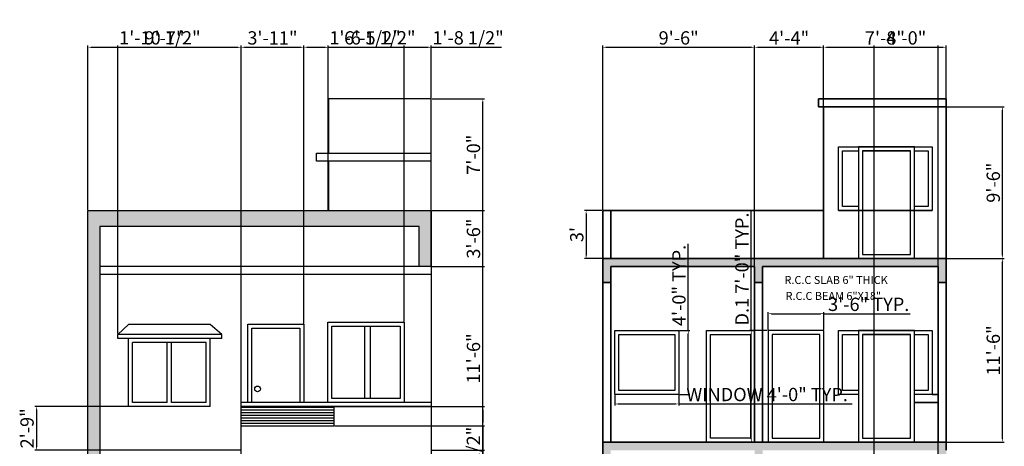
# Model space of a CAD drawing. Units: inches. Extents: x 2368 to 3882, y 1243 to 2139.
# Tile 6 of 6: x 3100 to 3840, y 1745 to 2065. Entities that reach past the tile are written whole.
import ezdxf

# ---------------------------------------------------------------- set-up
doc = ezdxf.new("R2010")
doc.units = ezdxf.units.IN
for name, color, linetype, lineweight in [('A-ANNO-DIMS', 2, 'Continuous', 18), ('A-ANNO-TEXT', 7, 'Continuous', 18), ('A-ELEV', 7, 'Continuous', 25), ('A-ELEV-PATT', 252, 'Continuous', 13), ('A-SECT', 7, 'Continuous', 35), ('A-SECT-PATT', 8, 'Continuous', 13)]:
    doc.layers.add(name, color=color, linetype=linetype, lineweight=lineweight)
doc.styles.get("Standard").update_dxf_attribs({"font": 'arial.ttf'})
doc.dimstyles.new('ISO-25', dxfattribs={"dimtxt": 10, "dimasz": 2.5, "dimexe": 1.25, "dimexo": 0.625, "dimtad": 1, "dimlunit": 3, "dimtxsty": 'Standard', "dimcen": 2.5, "dimadec": 0, "dimazin": 0, "dimtfac": 1, "dimtmove": 0, "dimatfit": 3, "dimfxl": 1, "dimarcsym": 0})

# ---------------------------------------------------------------- blocks, each defined once
blk = doc.blocks.new('*D13')
at = {"layer": 'A-ANNO-DIMS', "color": 0, "lineweight": -2, "transparency": 16777216}
for p, q in [((3537.71, 1921.84), (3524.56, 1921.84)), ((3525.81, 1919.34), (3525.81, 1888.34)), ((3537.71, 1885.84), (3524.56, 1885.84))]:
    blk.add_line(p, q, dxfattribs=at)
at = {"layer": 'A-ANNO-DIMS', "color": 0, "transparency": 16777216}
for points in [[(3525.39, 1919.34), (3526.22, 1919.34), (3525.81, 1921.84)], [(3525.39, 1888.34), (3526.22, 1888.34), (3525.81, 1885.84)]]:
    blk.add_solid(points, dxfattribs=at)
at = {"layer": 'Defpoints', "color": 0, "transparency": 16777216}
for p in [(3538.34, 1921.84), (3525.81, 1885.84), (3538.34, 1885.84)]:
    blk.add_point(p, dxfattribs=at)
at = {"layer": 'A-ANNO-DIMS', "color": 0, "transparency": 16777216, "insert": (3520.07, 1903.84), "char_height": 10, "attachment_point": 5, "rotation": 90}
blk.add_mtext("3'", dxfattribs=at)
blk = doc.blocks.new('WIN-ELEV-CHAJJA')
for p, q in [((3166.48, 1408.84), (3174.49, 1416.36)), ((3235.8, 1416.36), (3174.49, 1416.36)), ((3244.48, 1408.84), (3235.8, 1416.36)), ((3244.48, 1408.84), (3166.48, 1408.84)), ((3166.48, 1405.84), (3166.48, 1408.84)), ((3244.48, 1405.84), (3166.48, 1405.84)), ((3174.49, 1354.84), (3174.49, 1405.84)), ((3235.8, 1354.84), (3235.8, 1405.84)), ((3244.48, 1405.84), (3244.48, 1408.84)), ((3232.8, 1402.84), (3177.49, 1402.84)), ((3177.49, 1357.84), (3177.49, 1402.84)), ((3203.49, 1357.84), (3203.49, 1402.84)), ((3206.8, 1357.84), (3206.8, 1402.84)), ((3232.8, 1357.84), (3232.8, 1402.84)), ((3235.8, 1354.84), (3174.49, 1354.84)), ((3203.49, 1357.84), (3177.49, 1357.84)), ((3232.8, 1357.84), (3206.8, 1357.84))]:
    blk.add_line(p, q)
blk = doc.blocks.new('DOOR-ELEV')
for p, q in [((3271.73, 1507.84), (3271.73, 1566.55)), ((3271.73, 1566.55), (3313.73, 1566.55)), ((3274.73, 1507.84), (3274.73, 1563.55)), ((3274.73, 1563.55), (3310.73, 1563.55)), ((3310.73, 1563.55), (3310.73, 1507.84)), ((3313.73, 1566.55), (3313.73, 1507.84))]:
    blk.add_line(p, q)
blk.add_circle((3278.95, 1517.95), 2.15)
blk = doc.blocks.new('WIN-SECT-SQ')
for points in [[(3547.39, 1831.84), (3595.39, 1831.84), (3595.39, 1783.84), (3547.39, 1783.84)], [(3550.39, 1828.84), (3592.39, 1828.84), (3592.39, 1786.84), (3550.39, 1786.84)]]:
    blk.add_lwpolyline(points, close=True)
blk = doc.blocks.new('DOOR-SECT')
for points in [[(3662.52, 1747.84), (3704.52, 1747.84), (3704.52, 1831.84), (3662.52, 1831.84)], [(3665.52, 1750.84), (3701.52, 1750.84), (3701.52, 1828.84), (3665.52, 1828.84)]]:
    blk.add_lwpolyline(points, close=True)
blk = doc.blocks.new('DOOR-SECT-2')
for points in [[(3652.34, 1471.84), (3616.34, 1471.84), (3616.34, 1555.84), (3652.34, 1555.84)], [(3649.34, 1474.84), (3619.34, 1474.84), (3619.34, 1552.84), (3649.34, 1552.84)]]:
    blk.add_lwpolyline(points, close=True)
blk = doc.blocks.new('WIN-DOOR-SECT')
for points in [[(3730.54, 1783.84), (3715.45, 1783.84), (3715.45, 1831.84), (3785.77, 1831.84), (3785.77, 1783.84), (3772.54, 1783.84)], [(3730.54, 1786.84), (3718.45, 1786.84), (3718.45, 1828.84), (3730.54, 1828.84)], [(3733.54, 1828.84), (3769.54, 1828.84)], [(3772.54, 1828.84), (3782.77, 1828.84), (3782.77, 1786.84), (3772.54, 1786.84)]]:
    blk.add_lwpolyline(points)
for points in [[(3730.54, 1747.84), (3772.54, 1747.84), (3772.54, 1831.84), (3730.54, 1831.84)], [(3733.54, 1750.84), (3769.54, 1750.84), (3769.54, 1828.84), (3733.54, 1828.84)]]:
    blk.add_lwpolyline(points, close=True)
blk = doc.blocks.new('*D26')
at = {"layer": 'A-ANNO-DIMS', "color": 0, "lineweight": -2, "transparency": 16777216}
for p, q in [((3547.39, 1783.21), (3547.39, 1775.39)), ((3595.39, 1783.21), (3595.39, 1775.39)), ((3549.89, 1776.64), (3592.89, 1776.64)), ((3595.39, 1776.64), (3725.68, 1776.64))]:
    blk.add_line(p, q, dxfattribs=at)
at = {"layer": 'A-ANNO-DIMS', "color": 0, "transparency": 16777216}
for points in [[(3549.89, 1777.05), (3549.89, 1776.22), (3547.39, 1776.64)], [(3592.89, 1777.05), (3592.89, 1776.22), (3595.39, 1776.64)]]:
    blk.add_solid(points, dxfattribs=at)
at = {"layer": 'Defpoints', "color": 0, "transparency": 16777216}
for p in [(3547.39, 1783.84), (3595.39, 1783.84), (3595.39, 1776.64)]:
    blk.add_point(p, dxfattribs=at)
at = {"layer": 'A-ANNO-DIMS', "color": 0, "transparency": 16777216, "insert": (3661.79, 1782.44), "char_height": 10, "attachment_point": 5}
blk.add_mtext('WINDOW 4\'-0" TYP.', dxfattribs=at)
blk = doc.blocks.new('*D27')
at = {"layer": 'A-ANNO-DIMS', "color": 0, "lineweight": -2, "transparency": 16777216}
for p, q in [((3602.59, 1831.84), (3602.59, 1896.95)), ((3596.02, 1831.84), (3603.84, 1831.84)), ((3602.59, 1786.34), (3602.59, 1829.34)), ((3596.02, 1783.84), (3603.84, 1783.84))]:
    blk.add_line(p, q, dxfattribs=at)
at = {"layer": 'A-ANNO-DIMS', "color": 0, "transparency": 16777216}
for points in [[(3602.18, 1829.34), (3603.01, 1829.34), (3602.59, 1831.84)], [(3602.18, 1786.34), (3603.01, 1786.34), (3602.59, 1783.84)]]:
    blk.add_solid(points, dxfattribs=at)
at = {"layer": 'Defpoints', "color": 0, "transparency": 16777216}
for p in [(3595.39, 1831.84), (3602.59, 1831.84), (3595.39, 1783.84)]:
    blk.add_point(p, dxfattribs=at)
at = {"layer": 'A-ANNO-DIMS', "color": 0, "transparency": 16777216, "insert": (3596.86, 1865.64), "char_height": 10, "attachment_point": 5, "rotation": 90}
blk.add_mtext('4\'-0" TYP.', dxfattribs=at)
blk = doc.blocks.new('*D28')
at = {"layer": 'A-ANNO-DIMS', "color": 0, "lineweight": -2, "transparency": 16777216}
for p, q in [((3649.92, 1831.84), (3649.92, 1921.67)), ((3661.89, 1831.84), (3648.67, 1831.84)), ((3649.92, 1750.34), (3649.92, 1829.34)), ((3661.89, 1747.84), (3648.67, 1747.84))]:
    blk.add_line(p, q, dxfattribs=at)
at = {"layer": 'A-ANNO-DIMS', "color": 0, "transparency": 16777216}
for points in [[(3649.5, 1829.34), (3650.33, 1829.34), (3649.92, 1831.84)], [(3649.5, 1750.34), (3650.33, 1750.34), (3649.92, 1747.84)]]:
    blk.add_solid(points, dxfattribs=at)
at = {"layer": 'Defpoints', "color": 0, "transparency": 16777216}
for p in [(3649.92, 1831.84), (3662.52, 1831.84), (3662.52, 1747.84)]:
    blk.add_point(p, dxfattribs=at)
at = {"layer": 'A-ANNO-DIMS', "color": 0, "transparency": 16777216, "insert": (3644.19, 1878), "char_height": 10, "attachment_point": 5, "rotation": 90}
blk.add_mtext('D.1 7\'-0" TYP.', dxfattribs=at)
blk = doc.blocks.new('*D29')
at = {"layer": 'A-ANNO-DIMS', "color": 0, "lineweight": -2, "transparency": 16777216}
for p, q in [((3662.52, 1832.46), (3662.52, 1845.69)), ((3665.02, 1844.44), (3702.02, 1844.44)), ((3704.52, 1832.46), (3704.52, 1845.69)), ((3704.52, 1844.44), (3769.22, 1844.44))]:
    blk.add_line(p, q, dxfattribs=at)
at = {"layer": 'A-ANNO-DIMS', "color": 0, "transparency": 16777216}
for points in [[(3665.02, 1844.85), (3665.02, 1844.02), (3662.52, 1844.44)], [(3702.02, 1844.85), (3702.02, 1844.02), (3704.52, 1844.44)]]:
    blk.add_solid(points, dxfattribs=at)
at = {"layer": 'Defpoints', "color": 0, "transparency": 16777216}
for p in [(3704.52, 1844.44), (3662.52, 1831.84), (3704.52, 1831.84)]:
    blk.add_point(p, dxfattribs=at)
at = {"layer": 'A-ANNO-DIMS', "color": 0, "transparency": 16777216, "insert": (3738.12, 1850.17), "char_height": 10, "attachment_point": 5}
blk.add_mtext('3\'-6" TYP.', dxfattribs=at)
blk = doc.blocks.new('*D70')
at = {"layer": 'A-ANNO-DIMS', "color": 0, "lineweight": -2, "transparency": 16777216}
for p, q in [((3410.12, 1879.84), (3449.45, 1879.84)), ((3448.2, 1744.34), (3448.2, 1877.34)), ((3410.12, 1741.84), (3449.45, 1741.84))]:
    blk.add_line(p, q, dxfattribs=at)
at = {"layer": 'A-ANNO-DIMS', "color": 0, "transparency": 16777216}
for points in [[(3447.78, 1877.34), (3448.61, 1877.34), (3448.2, 1879.84)], [(3447.78, 1744.34), (3448.61, 1744.34), (3448.2, 1741.84)]]:
    blk.add_solid(points, dxfattribs=at)
at = {"layer": 'Defpoints', "color": 0, "transparency": 16777216}
for p in [(3409.5, 1879.84), (3448.2, 1879.84), (3409.5, 1741.84)]:
    blk.add_point(p, dxfattribs=at)
at = {"layer": 'A-ANNO-DIMS', "color": 0, "transparency": 16777216, "insert": (3442.47, 1810.84), "char_height": 10, "attachment_point": 5, "rotation": 90}
blk.add_mtext('11\'-6"', dxfattribs=at)
blk = doc.blocks.new('*D71')
at = {"layer": 'A-ANNO-DIMS', "color": 0, "lineweight": -2, "transparency": 16777216}
for p, q in [((3410.12, 1921.84), (3449.45, 1921.84)), ((3448.2, 1882.34), (3448.2, 1919.34)), ((3410.12, 1879.84), (3449.45, 1879.84))]:
    blk.add_line(p, q, dxfattribs=at)
at = {"layer": 'A-ANNO-DIMS', "color": 0, "transparency": 16777216}
for points in [[(3447.78, 1919.34), (3448.61, 1919.34), (3448.2, 1921.84)], [(3447.78, 1882.34), (3448.61, 1882.34), (3448.2, 1879.84)]]:
    blk.add_solid(points, dxfattribs=at)
at = {"layer": 'Defpoints', "color": 0, "transparency": 16777216}
for p in [(3409.5, 1921.84), (3448.2, 1921.84), (3409.5, 1879.84)]:
    blk.add_point(p, dxfattribs=at)
at = {"layer": 'A-ANNO-DIMS', "color": 0, "transparency": 16777216, "insert": (3442.46, 1900.84), "char_height": 10, "attachment_point": 5, "rotation": 90}
blk.add_mtext('3\'-6"', dxfattribs=at)
blk = doc.blocks.new('*D72')
at = {"layer": 'A-ANNO-DIMS', "color": 0, "lineweight": -2, "transparency": 16777216}
for p, q in [((3410.12, 2005.84), (3449.45, 2005.84)), ((3448.2, 1924.34), (3448.2, 2003.34)), ((3410.12, 1921.84), (3449.45, 1921.84))]:
    blk.add_line(p, q, dxfattribs=at)
at = {"layer": 'A-ANNO-DIMS', "color": 0, "transparency": 16777216}
for points in [[(3447.78, 2003.34), (3448.61, 2003.34), (3448.2, 2005.84)], [(3447.78, 1924.34), (3448.61, 1924.34), (3448.2, 1921.84)]]:
    blk.add_solid(points, dxfattribs=at)
at = {"layer": 'Defpoints', "color": 0, "transparency": 16777216}
for p in [(3409.5, 2005.84), (3448.2, 2005.84), (3409.5, 1921.84)]:
    blk.add_point(p, dxfattribs=at)
at = {"layer": 'A-ANNO-DIMS', "color": 0, "transparency": 16777216, "insert": (3442.47, 1963.84), "char_height": 10, "attachment_point": 5, "rotation": 90}
blk.add_mtext('7\'-0"', dxfattribs=at)
blk = doc.blocks.new('*D73')
at = {"layer": 'A-ANNO-DIMS', "color": 0, "lineweight": -2, "transparency": 16777216}
for p, q in [((3410.12, 2005.84), (3449.45, 2005.84)), ((3448.2, 1297.34), (3448.2, 2003.34)), ((3410.12, 1294.84), (3449.45, 1294.84))]:
    blk.add_line(p, q, dxfattribs=at)
at = {"layer": 'A-ANNO-DIMS', "color": 0, "transparency": 16777216}
for points in [[(3447.78, 2003.34), (3448.61, 2003.34), (3448.2, 2005.84)], [(3447.78, 1297.34), (3448.61, 1297.34), (3448.2, 1294.84)]]:
    blk.add_solid(points, dxfattribs=at)
at = {"layer": 'Defpoints', "color": 0, "transparency": 16777216}
for p in [(3409.5, 2005.84), (3448.2, 2005.84), (3409.5, 1294.84)]:
    blk.add_point(p, dxfattribs=at)
at = {"layer": 'A-ANNO-DIMS', "color": 0, "transparency": 16777216, "insert": (3442.46, 1650.34), "char_height": 10, "attachment_point": 5, "rotation": 90}
blk.add_mtext('59\'-3"', dxfattribs=at)
blk = doc.blocks.new('*D74')
at = {"layer": 'A-ANNO-DIMS', "color": 0, "lineweight": -2, "transparency": 16777216}
for p, q in [((3151.5, 1922.46), (3151.5, 2045.79)), ((3154, 2044.54), (3264.09, 2044.54)), ((3266.59, 1874.46), (3266.59, 2045.79))]:
    blk.add_line(p, q, dxfattribs=at)
at = {"layer": 'A-ANNO-DIMS', "color": 0, "transparency": 16777216}
for points in [[(3154, 2044.95), (3154, 2044.12), (3151.5, 2044.54)], [(3264.09, 2044.95), (3264.09, 2044.12), (3266.59, 2044.54)]]:
    blk.add_solid(points, dxfattribs=at)
at = {"layer": 'Defpoints', "color": 0, "transparency": 16777216}
for p in [(3266.59, 2044.54), (3151.5, 1921.84), (3266.59, 1873.84)]:
    blk.add_point(p, dxfattribs=at)
at = {"layer": 'A-ANNO-DIMS', "color": 0, "transparency": 16777216, "insert": (3209.04, 2050.27), "char_height": 10, "attachment_point": 5}
blk.add_mtext('9\'-7"', dxfattribs=at)
blk = doc.blocks.new('*D75')
at = {"layer": 'A-ANNO-DIMS', "color": 0, "lineweight": -2, "transparency": 16777216}
for p, q in [((3266.59, 1874.46), (3266.59, 2045.79)), ((3269.09, 2044.54), (3311.23, 2044.54)), ((3313.73, 1837.17), (3313.73, 2045.79))]:
    blk.add_line(p, q, dxfattribs=at)
at = {"layer": 'A-ANNO-DIMS', "color": 0, "transparency": 16777216}
for points in [[(3269.09, 2044.95), (3269.09, 2044.12), (3266.59, 2044.54)], [(3311.23, 2044.95), (3311.23, 2044.12), (3313.73, 2044.54)]]:
    blk.add_solid(points, dxfattribs=at)
at = {"layer": 'Defpoints', "color": 0, "transparency": 16777216}
for p in [(3313.73, 2044.54), (3266.59, 1873.84), (3313.73, 1836.55)]:
    blk.add_point(p, dxfattribs=at)
at = {"layer": 'A-ANNO-DIMS', "color": 0, "transparency": 16777216, "insert": (3290.16, 2050.27), "char_height": 10, "attachment_point": 5}
blk.add_mtext('3\'-11"', dxfattribs=at)
blk = doc.blocks.new('*D76')
at = {"layer": 'A-ANNO-DIMS', "color": 0, "lineweight": -2, "transparency": 16777216}
for p, q in [((3313.73, 1837.17), (3313.73, 2045.79)), ((3316.23, 2044.54), (3329.63, 2044.54)), ((3332.13, 1922.46), (3332.13, 2045.79)), ((3332.13, 2044.54), (3384.83, 2044.54))]:
    blk.add_line(p, q, dxfattribs=at)
at = {"layer": 'A-ANNO-DIMS', "color": 0, "transparency": 16777216}
for points in [[(3316.23, 2044.95), (3316.23, 2044.12), (3313.73, 2044.54)], [(3329.63, 2044.95), (3329.63, 2044.12), (3332.13, 2044.54)]]:
    blk.add_solid(points, dxfattribs=at)
at = {"layer": 'Defpoints', "color": 0, "transparency": 16777216}
for p in [(3332.13, 2044.54), (3332.13, 1921.84), (3313.73, 1836.55)]:
    blk.add_point(p, dxfattribs=at)
at = {"layer": 'A-ANNO-DIMS', "color": 0, "transparency": 16777216, "insert": (3359.73, 2050.33), "char_height": 10, "attachment_point": 5}
blk.add_mtext('1\'-6 1/2"', dxfattribs=at)
blk = doc.blocks.new('*D77')
at = {"layer": 'A-ANNO-DIMS', "color": 0, "lineweight": -2, "transparency": 16777216}
for p, q in [((3332.13, 2006.46), (3332.13, 2045.79)), ((3334.63, 2044.54), (3407, 2044.54)), ((3409.5, 2006.46), (3409.5, 2045.79))]:
    blk.add_line(p, q, dxfattribs=at)
at = {"layer": 'A-ANNO-DIMS', "color": 0, "transparency": 16777216}
for points in [[(3334.63, 2044.95), (3334.63, 2044.12), (3332.13, 2044.54)], [(3407, 2044.95), (3407, 2044.12), (3409.5, 2044.54)]]:
    blk.add_solid(points, dxfattribs=at)
at = {"layer": 'Defpoints', "color": 0, "transparency": 16777216}
for p in [(3409.5, 2044.54), (3332.13, 2005.84), (3409.5, 2005.84)]:
    blk.add_point(p, dxfattribs=at)
at = {"layer": 'A-ANNO-DIMS', "color": 0, "transparency": 16777216, "insert": (3370.82, 2050.33), "char_height": 10, "attachment_point": 5}
blk.add_mtext('6\'-5 1/2"', dxfattribs=at)
blk = doc.blocks.new('*D78')
at = {"layer": 'A-ANNO-DIMS', "color": 0, "lineweight": -2, "transparency": 16777216}
for p, q in [((3151.5, 1922.46), (3151.5, 2045.79)), ((3154, 2044.54), (3171.6, 2044.54)), ((3174.1, 1829.46), (3174.1, 2045.79)), ((3174.1, 2044.54), (3234.56, 2044.54))]:
    blk.add_line(p, q, dxfattribs=at)
at = {"layer": 'A-ANNO-DIMS', "color": 0, "transparency": 16777216}
for points in [[(3154, 2044.95), (3154, 2044.12), (3151.5, 2044.54)], [(3171.6, 2044.95), (3171.6, 2044.12), (3174.1, 2044.54)]]:
    blk.add_solid(points, dxfattribs=at)
at = {"layer": 'Defpoints', "color": 0, "transparency": 16777216}
for p in [(3174.1, 2044.54), (3151.5, 1921.84), (3174.1, 1828.84)]:
    blk.add_point(p, dxfattribs=at)
at = {"layer": 'A-ANNO-DIMS', "color": 0, "transparency": 16777216, "insert": (3205.58, 2050.33), "char_height": 10, "attachment_point": 5}
blk.add_mtext('1\'-10 1/2"', dxfattribs=at)
blk = doc.blocks.new('*D79')
at = {"layer": 'A-ANNO-DIMS', "color": 0, "lineweight": -2, "transparency": 16777216}
for p, q in [((3389.04, 1838.65), (3389.04, 2045.79)), ((3391.54, 2044.54), (3407, 2044.54)), ((3409.5, 1880.46), (3409.5, 2045.79)), ((3409.5, 2044.54), (3462.19, 2044.54))]:
    blk.add_line(p, q, dxfattribs=at)
at = {"layer": 'A-ANNO-DIMS', "color": 0, "transparency": 16777216}
for points in [[(3391.54, 2044.95), (3391.54, 2044.12), (3389.04, 2044.54)], [(3407, 2044.95), (3407, 2044.12), (3409.5, 2044.54)]]:
    blk.add_solid(points, dxfattribs=at)
at = {"layer": 'Defpoints', "color": 0, "transparency": 16777216}
for p in [(3409.5, 2044.54), (3409.5, 1879.84), (3389.04, 1838.02)]:
    blk.add_point(p, dxfattribs=at)
at = {"layer": 'A-ANNO-DIMS', "color": 0, "transparency": 16777216, "insert": (3437.09, 2050.33), "char_height": 10, "attachment_point": 5}
blk.add_mtext('1\'-8 1/2"', dxfattribs=at)
blk = doc.blocks.new('*D80')
at = {"layer": 'A-ANNO-DIMS', "color": 0, "lineweight": -2, "transparency": 16777216}
for p, q in [((3242.81, 1774.84), (3111.55, 1774.84)), ((3112.8, 1772.34), (3112.8, 1744.34)), ((3265.97, 1741.84), (3111.55, 1741.84))]:
    blk.add_line(p, q, dxfattribs=at)
at = {"layer": 'A-ANNO-DIMS', "color": 0, "transparency": 16777216}
for points in [[(3112.38, 1772.34), (3113.21, 1772.34), (3112.8, 1774.84)], [(3112.38, 1744.34), (3113.21, 1744.34), (3112.8, 1741.84)]]:
    blk.add_solid(points, dxfattribs=at)
at = {"layer": 'Defpoints', "color": 0, "transparency": 16777216}
for p in [(3243.43, 1774.84), (3112.8, 1741.84), (3266.59, 1741.84)]:
    blk.add_point(p, dxfattribs=at)
at = {"layer": 'A-ANNO-DIMS', "color": 0, "transparency": 16777216, "insert": (3107.07, 1758.34), "char_height": 10, "attachment_point": 5, "rotation": 90}
blk.add_mtext('2\'-9"', dxfattribs=at)
blk = doc.blocks.new('*D81')
at = {"layer": 'A-ANNO-DIMS', "color": 0, "lineweight": -2, "transparency": 16777216}
for p, q in [((3337.1, 1774.84), (3449.45, 1774.84)), ((3448.2, 1772.34), (3448.2, 1762.79)), ((3337.1, 1760.29), (3449.45, 1760.29)), ((3448.2, 1760.29), (3448.2, 1707.6))]:
    blk.add_line(p, q, dxfattribs=at)
at = {"layer": 'A-ANNO-DIMS', "color": 0, "transparency": 16777216}
for points in [[(3447.78, 1772.34), (3448.61, 1772.34), (3448.2, 1774.84)], [(3447.78, 1762.79), (3448.61, 1762.79), (3448.2, 1760.29)]]:
    blk.add_solid(points, dxfattribs=at)
at = {"layer": 'Defpoints', "color": 0, "transparency": 16777216}
for p in [(3336.47, 1774.84), (3336.47, 1760.29), (3448.2, 1760.29)]:
    blk.add_point(p, dxfattribs=at)
at = {"layer": 'A-ANNO-DIMS', "color": 0, "transparency": 16777216, "insert": (3442.4, 1732.69), "char_height": 10, "attachment_point": 5, "rotation": 90}
blk.add_mtext('1\'-2 1/2"', dxfattribs=at)
blk = doc.blocks.new('*D87')
at = {"layer": 'A-ANNO-DIMS', "color": 0, "lineweight": -2, "transparency": 16777216}
for p, q in [((3538.34, 1922.46), (3538.34, 2045.79)), ((3540.84, 2044.54), (3649.84, 2044.54)), ((3652.34, 1880.46), (3652.34, 2045.79))]:
    blk.add_line(p, q, dxfattribs=at)
at = {"layer": 'A-ANNO-DIMS', "color": 0, "transparency": 16777216}
for points in [[(3540.84, 2044.95), (3540.84, 2044.12), (3538.34, 2044.54)], [(3649.84, 2044.95), (3649.84, 2044.12), (3652.34, 2044.54)]]:
    blk.add_solid(points, dxfattribs=at)
at = {"layer": 'Defpoints', "color": 0, "transparency": 16777216}
for p in [(3652.34, 2044.54), (3538.34, 1921.84), (3652.34, 1879.84)]:
    blk.add_point(p, dxfattribs=at)
at = {"layer": 'A-ANNO-DIMS', "color": 0, "transparency": 16777216, "insert": (3595.34, 2050.27), "char_height": 10, "attachment_point": 5}
blk.add_mtext('9\'-6"', dxfattribs=at)
blk = doc.blocks.new('*D88')
at = {"layer": 'A-ANNO-DIMS', "color": 0, "lineweight": -2, "transparency": 16777216}
for p, q in [((3652.34, 1880.46), (3652.34, 2045.79)), ((3654.84, 2044.54), (3701.77, 2044.54)), ((3704.27, 1922.46), (3704.27, 2045.79))]:
    blk.add_line(p, q, dxfattribs=at)
at = {"layer": 'A-ANNO-DIMS', "color": 0, "transparency": 16777216}
for points in [[(3654.84, 2044.95), (3654.84, 2044.12), (3652.34, 2044.54)], [(3701.77, 2044.95), (3701.77, 2044.12), (3704.27, 2044.54)]]:
    blk.add_solid(points, dxfattribs=at)
at = {"layer": 'Defpoints', "color": 0, "transparency": 16777216}
for p in [(3704.27, 2044.54), (3704.27, 1921.84), (3652.34, 1879.84)]:
    blk.add_point(p, dxfattribs=at)
at = {"layer": 'A-ANNO-DIMS', "color": 0, "transparency": 16777216, "insert": (3678.31, 2050.16), "char_height": 10, "attachment_point": 5}
blk.add_mtext('4\'-4"', dxfattribs=at)
blk = doc.blocks.new('*D89')
at = {"layer": 'A-ANNO-DIMS', "color": 0, "lineweight": -2, "transparency": 16777216}
for p, q in [((3704.27, 2000.46), (3704.27, 2045.79)), ((3706.77, 2044.54), (3793.84, 2044.54)), ((3796.34, 2000.46), (3796.34, 2045.79))]:
    blk.add_line(p, q, dxfattribs=at)
at = {"layer": 'A-ANNO-DIMS', "color": 0, "transparency": 16777216}
for points in [[(3706.77, 2044.95), (3706.77, 2044.12), (3704.27, 2044.54)], [(3793.84, 2044.95), (3793.84, 2044.12), (3796.34, 2044.54)]]:
    blk.add_solid(points, dxfattribs=at)
at = {"layer": 'Defpoints', "color": 0, "transparency": 16777216}
for p in [(3796.34, 2044.54), (3704.27, 1999.84), (3796.34, 1999.84)]:
    blk.add_point(p, dxfattribs=at)
at = {"layer": 'A-ANNO-DIMS', "color": 0, "transparency": 16777216, "insert": (3750.31, 2050.27), "char_height": 10, "attachment_point": 5}
blk.add_mtext('7\'-8"', dxfattribs=at)
blk = doc.blocks.new('*D90')
at = {"layer": 'A-ANNO-DIMS', "color": 0, "lineweight": -2, "transparency": 16777216}
for p, q in [((3796.96, 1999.84), (3839.99, 1999.84)), ((3838.74, 1888.34), (3838.74, 1997.34)), ((3796.96, 1885.84), (3839.99, 1885.84))]:
    blk.add_line(p, q, dxfattribs=at)
at = {"layer": 'A-ANNO-DIMS', "color": 0, "transparency": 16777216}
for points in [[(3838.33, 1997.34), (3839.16, 1997.34), (3838.74, 1999.84)], [(3838.33, 1888.34), (3839.16, 1888.34), (3838.74, 1885.84)]]:
    blk.add_solid(points, dxfattribs=at)
at = {"layer": 'Defpoints', "color": 0, "transparency": 16777216}
for p in [(3796.34, 1999.84), (3838.74, 1999.84), (3796.34, 1885.84)]:
    blk.add_point(p, dxfattribs=at)
at = {"layer": 'A-ANNO-DIMS', "color": 0, "transparency": 16777216, "insert": (3833.01, 1942.84), "char_height": 10, "attachment_point": 5, "rotation": 90}
blk.add_mtext('9\'-6"', dxfattribs=at)
blk = doc.blocks.new('*D91')
at = {"layer": 'A-ANNO-DIMS', "color": 0, "lineweight": -2, "transparency": 16777216}
for p, q in [((3796.96, 1885.84), (3839.99, 1885.84)), ((3838.74, 1750.34), (3838.74, 1883.34)), ((3796.96, 1747.84), (3839.99, 1747.84))]:
    blk.add_line(p, q, dxfattribs=at)
at = {"layer": 'A-ANNO-DIMS', "color": 0, "transparency": 16777216}
for points in [[(3838.33, 1883.34), (3839.16, 1883.34), (3838.74, 1885.84)], [(3838.33, 1750.34), (3839.16, 1750.34), (3838.74, 1747.84)]]:
    blk.add_solid(points, dxfattribs=at)
at = {"layer": 'Defpoints', "color": 0, "transparency": 16777216}
for p in [(3796.34, 1885.84), (3838.74, 1885.84), (3796.34, 1747.84)]:
    blk.add_point(p, dxfattribs=at)
at = {"layer": 'A-ANNO-DIMS', "color": 0, "transparency": 16777216, "insert": (3833.01, 1816.84), "char_height": 10, "attachment_point": 5, "rotation": 90}
blk.add_mtext('11\'-6"', dxfattribs=at)
blk = doc.blocks.new('*D94')
at = {"layer": 'A-ANNO-DIMS', "color": 0, "lineweight": -2, "transparency": 16777216}
for p, q in [((3742.34, 1388.46), (3742.34, 2045.79)), ((3744.84, 2044.54), (3787.84, 2044.54)), ((3790.34, 1388.46), (3790.34, 2045.79))]:
    blk.add_line(p, q, dxfattribs=at)
at = {"layer": 'A-ANNO-DIMS', "color": 0, "transparency": 16777216}
for points in [[(3744.84, 2044.95), (3744.84, 2044.12), (3742.34, 2044.54)], [(3787.84, 2044.95), (3787.84, 2044.12), (3790.34, 2044.54)]]:
    blk.add_solid(points, dxfattribs=at)
at = {"layer": 'Defpoints', "color": 0, "transparency": 16777216}
for p in [(3790.34, 2044.54), (3742.34, 1387.84), (3790.34, 1387.84)]:
    blk.add_point(p, dxfattribs=at)
at = {"layer": 'A-ANNO-DIMS', "color": 0, "transparency": 16777216, "insert": (3766.34, 2050.27), "char_height": 10, "attachment_point": 5}
blk.add_mtext('4\'-0"', dxfattribs=at)

msp = doc.modelspace()

# ---------------------------------------------------------------- hatches: boundary and pattern name
at = {"layer": 'A-ELEV-PATT'}
h = msp.add_hatch(dxfattribs=at)
h.set_pattern_fill('AR-CONC', color=256, scale=0.066)
h.paths.add_polyline_path([(3409.496, 1921.838), (3151.496, 1921.838), (3151.496, 1471.838), (3160.496, 1471.838), (3160.496, 1909.838), (3400.496, 1909.838), (3400.496, 1879.838), (3409.496, 1879.838)])
at = {"layer": 'A-SECT-PATT'}
h = msp.add_hatch(color=256, dxfattribs=at)
h.dxf.hatch_style = 1
h.paths.add_polyline_path([(3796.338, 1321.838), (3538.338, 1321.838), (3538.338, 1315.838), (3796.338, 1315.838)])
h.paths.add_polyline_path([(3796.338, 1471.838), (3538.338, 1471.838), (3538.338, 1453.838), (3544.338, 1453.838), (3544.338, 1465.838), (3736.338, 1465.838), (3736.338, 1453.838), (3742.338, 1453.838), (3742.338, 1465.838), (3790.338, 1465.838), (3790.338, 1453.838), (3796.338, 1453.838), (3796.338, 1465.838)])
h.paths.add_polyline_path([(3796.338, 1609.838), (3538.338, 1609.838), (3538.338, 1591.838), (3544.338, 1591.838), (3544.338, 1603.838), (3652.338, 1603.838), (3652.338, 1591.838), (3658.338, 1591.838), (3658.338, 1603.838), (3790.338, 1603.838), (3790.338, 1591.838), (3796.338, 1591.838), (3796.338, 1603.838)])
h.paths.add_polyline_path([(3796.338, 1747.838), (3538.338, 1747.838), (3538.338, 1729.838), (3544.338, 1729.838), (3544.338, 1741.838), (3652.338, 1741.838), (3652.338, 1729.838), (3658.338, 1729.838), (3658.338, 1741.838), (3790.338, 1741.838), (3790.338, 1729.838), (3796.338, 1729.838), (3796.338, 1741.838)])
h.paths.add_polyline_path([(3796.338, 1885.838), (3538.338, 1885.838), (3538.338, 1867.838), (3544.338, 1867.838), (3544.338, 1879.838), (3652.338, 1879.838), (3652.338, 1867.838), (3658.338, 1867.838), (3658.338, 1879.838), (3790.338, 1879.838), (3790.338, 1867.838), (3796.338, 1867.838), (3796.338, 1879.838)])

# ---------------------------------------------------------------- linework, layer by layer
at = {"layer": 'A-ELEV'}
for p, q in [((3409.496, 2005.838), (3332.134, 2005.838)), ((3332.134, 2005.838), (3332.134, 1965.082)), ((3409.496, 1921.838), (3409.496, 2005.838)), ((3323.299, 1959.082), (3323.299, 1965.082)), ((3323.299, 1965.082), (3409.496, 1965.082)), ((3409.496, 1959.082), (3323.299, 1959.082)), ((3332.134, 1959.082), (3332.134, 1921.838)), ((3151.496, 1294.838), (3151.496, 1921.838)), ((3151.496, 1921.838), (3409.496, 1921.838)), ((3409.496, 1921.838), (3409.496, 1294.838)), ((3400.496, 1909.838), (3160.496, 1909.838)), ((3160.496, 1909.838), (3160.496, 1471.838)), ((3400.496, 1879.838), (3400.496, 1909.838)), ((3409.496, 1879.838), (3160.496, 1879.838)), ((3409.496, 1879.838), (3400.496, 1879.838)), ((3409.496, 1879.838), (3409.496, 1879.838)), ((3409.496, 1873.838), (3160.496, 1873.838)), ((3266.593, 1471.838), (3266.593, 1873.838)), ((3359.418, 1835.025), (3359.418, 1780.838)), ((3363.593, 1835.025), (3363.593, 1780.838)), ((3409.496, 1777.838), (3266.593, 1777.838)), ((3409.496, 1774.838), (3266.593, 1774.838)), ((3266.593, 1774.289), (3336.475, 1774.289)), ((3266.593, 1772.289), (3336.475, 1772.289)), ((3266.593, 1770.289), (3336.475, 1770.289)), ((3266.593, 1768.289), (3336.475, 1768.289)), ((3336.475, 1760.289), (3336.475, 1774.838)), ((3266.593, 1766.289), (3336.475, 1766.289)), ((3266.593, 1764.289), (3336.475, 1764.289)), ((3266.593, 1762.289), (3336.475, 1762.289)), ((3266.593, 1760.289), (3336.475, 1760.289))]:
    msp.add_line(p, q, dxfattribs=at)
for points in [[(3331.795, 1838.025), (3389.041, 1838.025), (3389.041, 1777.838), (3331.795, 1777.838)], [(3334.795, 1835.025), (3386.041, 1835.025), (3386.041, 1780.838), (3334.795, 1780.838)]]:
    msp.add_lwpolyline(points, close=True, dxfattribs=at)
at = {"layer": 'A-SECT'}
for p, q in [((3796.338, 2005.838), (3700.338, 2005.838)), ((3700.338, 2005.838), (3700.338, 1999.838)), ((3796.338, 1885.838), (3796.338, 2005.838)), ((3700.338, 1999.838), (3796.338, 1999.838)), ((3704.274, 1999.838), (3704.274, 1885.838)), ((3538.338, 1885.838), (3538.338, 1921.838)), ((3538.338, 1921.838), (3704.274, 1921.838)), ((3544.338, 1885.838), (3544.338, 1921.838)), ((3715.454, 1921.838), (3785.773, 1921.838)), ((3538.338, 1747.838), (3538.338, 1885.838)), ((3796.338, 1885.838), (3538.338, 1885.838)), ((3544.338, 1879.838), (3652.338, 1879.838)), ((3544.338, 1747.838), (3544.338, 1879.838)), ((3652.338, 1747.838), (3652.338, 1879.838)), ((3658.338, 1747.838), (3658.338, 1879.838)), ((3658.338, 1879.838), (3790.338, 1879.838)), ((3790.338, 1747.838), (3790.338, 1879.838)), ((3796.338, 1879.838), (3796.338, 1885.838)), ((3796.338, 1747.838), (3796.338, 1879.838)), ((3544.338, 1867.838), (3538.338, 1867.838)), ((3658.338, 1867.838), (3652.338, 1867.838)), ((3796.338, 1867.838), (3790.338, 1867.838)), ((3785.773, 1783.838), (3790.338, 1783.838)), ((3772.538, 1777.838), (3790.338, 1777.838)), ((3538.338, 1609.838), (3538.338, 1747.838)), ((3796.338, 1747.838), (3538.338, 1747.838)), ((3796.338, 1741.838), (3796.338, 1747.838))]:
    msp.add_line(p, q, dxfattribs=at)

# ---------------------------------------------------------------- block references
at = {"layer": 'A-ELEV'}
for name, p in [('WIN-DOOR-SECT', (0, 138)), ('WIN-ELEV-CHAJJA', (7.627, 420)), ('DOOR-ELEV', (0, 270)), ('WIN-SECT-SQ', (0, 0)), ('DOOR-SECT-2', (0, 276)), ('DOOR-SECT', (0, 0)), ('WIN-DOOR-SECT', (0, 0))]:
    msp.add_blockref(name, p, dxfattribs=at)

# ---------------------------------------------------------------- texts
at = {"layer": 'A-ANNO-TEXT'}
for s, p in [('R.C.C SLAB 6" THICK', (3674.843, 1866.742)), ('R.C.C BEAM 6"X18"', (3675.66, 1854.764))]:
    msp.add_text(s, height=6, dxfattribs=at).set_placement(p)

# ---------------------------------------------------------------- dimensions: what is measured, and where the dimension line sits
at = {"layer": 'A-ANNO-DIMS'}
for base, p1, p2, picture, middle in [((3174.102, 2044.538), (3151.496, 1921.838), (3174.102, 1828.838), '*D78', (3205.583, 2050.333)), ((3332.134, 2044.538), (3313.728, 1836.546), (3332.134, 1921.838), '*D76', (3359.731, 2050.333)), ((3409.496, 2044.538), (3332.134, 2005.838), (3409.496, 2005.838), '*D77', (3370.815, 2050.333)), ((3409.496, 2044.538), (3389.041, 1838.025), (3409.496, 1879.838), '*D79', (3437.093, 2050.333)), ((3266.593, 2044.538), (3151.496, 1921.838), (3266.593, 1873.838), '*D74', (3209.045, 2050.268)), ((3313.728, 2044.538), (3266.593, 1873.838), (3313.728, 1836.546), '*D75', (3290.16, 2050.272)), ((3652.338, 2044.538), (3538.338, 1921.838), (3652.338, 1879.838), '*D87', (3595.338, 2050.268)), ((3704.274, 2044.538), (3652.338, 1879.838), (3704.274, 1921.838), '*D88', (3678.306, 2050.163)), ((3796.338, 2044.538), (3704.274, 1999.838), (3796.338, 1999.838), '*D89', (3750.306, 2050.268)), ((3790.338, 2044.538), (3742.338, 1387.838), (3790.338, 1387.838), '*D94', (3766.338, 2050.268))]:
    dim = msp.add_linear_dim(base=base, p1=p1, p2=p2, dimstyle='ISO-25', override={"dimdec": 1, "dimlfac": 1, "dimrnd": 0, "dimzin": 1, "dimdsep": 46, "dimlunit": 4, "dimfrac": 2}, dxfattribs=at)
    dim.commit()
    dim.dimension.update_dxf_attribs({"geometry": picture, "text_midpoint": middle})
for base, p1, p2, override, picture, middle in [((3448.196, 2005.838), (3409.496, 1921.838), (3409.496, 2005.838), {"dimdec": 1, "dimlfac": 1, "dimrnd": 0, "dimzin": 1, "dimdsep": 46, "dimlunit": 4, "dimfrac": 2}, '*D72', (3442.466, 1963.838)), ((3448.196, 2005.838), (3409.496, 1294.838), (3409.496, 2005.838), {"dimdec": 1, "dimlfac": 1, "dimrnd": 0, "dimzin": 1, "dimdsep": 46, "dimlunit": 4, "dimfrac": 2}, '*D73', (3442.462, 1650.338)), ((3838.744, 1999.838), (3796.338, 1885.838), (3796.338, 1999.838), {"dimdec": 1, "dimlfac": 1, "dimrnd": 0, "dimzin": 1, "dimdsep": 46, "dimlunit": 4, "dimfrac": 2}, '*D90', (3833.013, 1942.838)), ((3448.196, 1921.838), (3409.496, 1879.838), (3409.496, 1921.838), {"dimdec": 1, "dimlfac": 1, "dimrnd": 0, "dimzin": 1, "dimdsep": 46, "dimlunit": 4, "dimfrac": 2}, '*D71', (3442.462, 1900.838)), ((3525.807, 1885.838), (3538.338, 1921.838), (3538.338, 1885.838), {"dimclrd": 0, "dimclre": 0, "dimclrt": 0}, '*D13', (3520.073, 1903.838)), ((3448.196, 1879.838), (3409.496, 1741.838), (3409.496, 1879.838), {"dimdec": 1, "dimlfac": 1, "dimrnd": 0, "dimzin": 1, "dimdsep": 46, "dimlunit": 4, "dimfrac": 2}, '*D70', (3442.466, 1810.838)), ((3838.744, 1885.838), (3796.338, 1747.838), (3796.338, 1885.838), {"dimdec": 1, "dimlfac": 1, "dimrnd": 0, "dimzin": 1, "dimdsep": 46, "dimlunit": 4, "dimfrac": 2}, '*D91', (3833.013, 1816.838)), ((3112.796, 1741.838), (3243.431, 1774.838), (3266.593, 1741.838), {"dimdec": 1, "dimlfac": 1, "dimrnd": 0, "dimzin": 1, "dimdsep": 46, "dimlunit": 4, "dimfrac": 2}, '*D80', (3107.066, 1758.338)), ((3448.196, 1760.289), (3336.475, 1774.838), (3336.475, 1760.289), {"dimdec": 1, "dimlfac": 1, "dimrnd": 0, "dimzin": 1, "dimdsep": 46, "dimlunit": 4, "dimfrac": 2}, '*D81', (3442.401, 1732.692))]:
    dim = msp.add_linear_dim(base=base, p1=p1, p2=p2, angle=90, dimstyle='ISO-25', override=override, dxfattribs=at)
    dim.commit()
    dim.dimension.update_dxf_attribs({"geometry": picture, "text_midpoint": middle})
for base, p1, p2, text, picture, middle in [((3649.917, 1831.838), (3662.517, 1747.838), (3662.517, 1831.838), 'D.1 <> TYP.', '*D28', (3644.186, 1878.002)), ((3602.593, 1831.838), (3595.393, 1783.838), (3595.393, 1831.838), '<> TYP.', '*D27', (3596.862, 1865.641))]:
    dim = msp.add_linear_dim(base=base, p1=p1, p2=p2, angle=90, text=text, dimstyle='ISO-25', override={"dimdec": 1, "dimrnd": 0, "dimzin": 1, "dimlunit": 4, "dimfrac": 2}, dxfattribs=at)
    dim.commit()
    dim.dimension.update_dxf_attribs({"geometry": picture, "text_midpoint": middle})
for base, p1, p2, text, picture, middle in [((3704.517, 1844.438), (3662.517, 1831.838), (3704.517, 1831.838), '<> TYP.', '*D29', (3738.116, 1850.172)), ((3595.393, 1776.638), (3547.393, 1783.838), (3595.393, 1783.838), 'WINDOW <> TYP.', '*D26', (3661.789, 1782.437))]:
    dim = msp.add_linear_dim(base=base, p1=p1, p2=p2, text=text, dimstyle='ISO-25', override={"dimdec": 1, "dimrnd": 0, "dimzin": 1, "dimlunit": 4, "dimfrac": 2}, dxfattribs=at)
    dim.commit()
    dim.dimension.update_dxf_attribs({"geometry": picture, "text_midpoint": middle})

doc.saveas('drawing.dxf')
